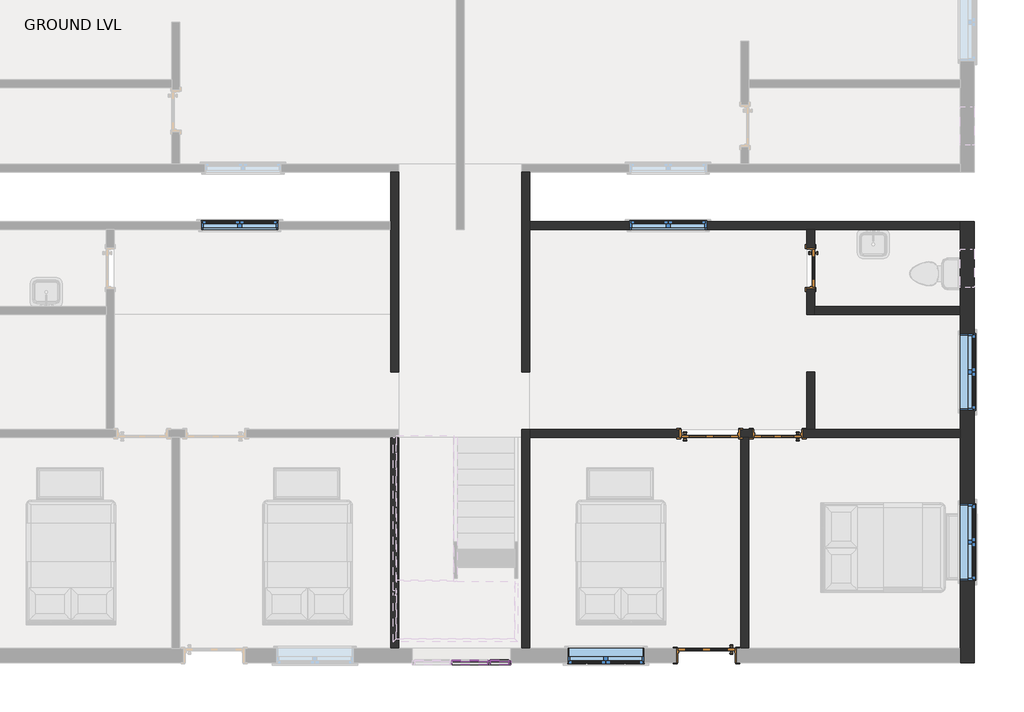
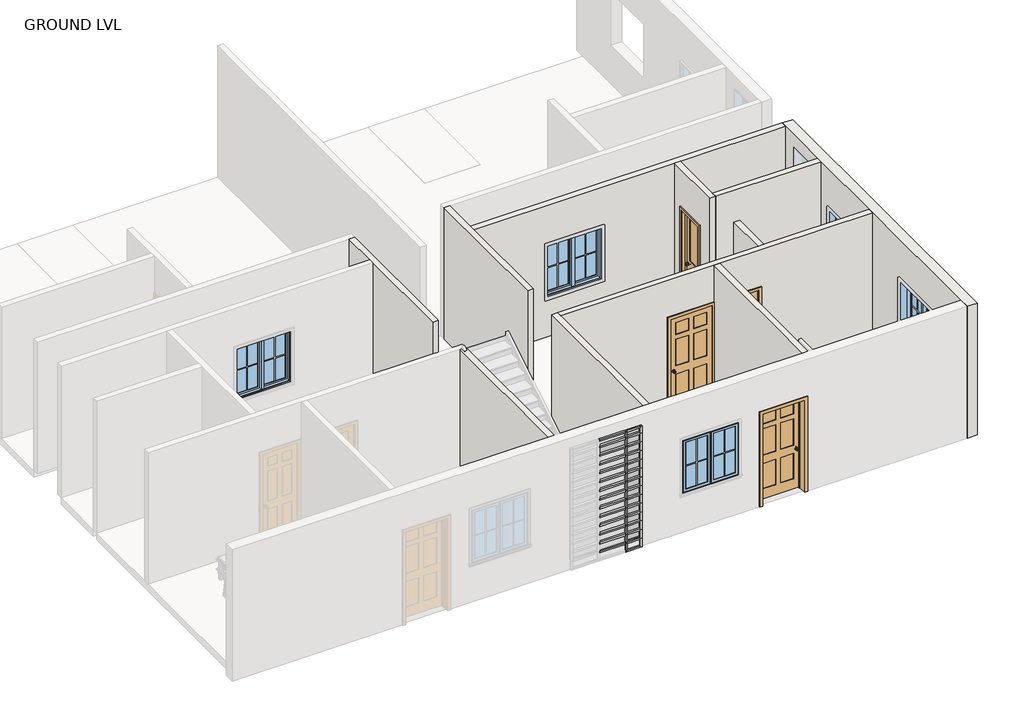
# One storey, part 2 of 4: 57 members, 15 plates, 11 walls, 5 windows, 4 doors.
"""IFC4 building model written with IfcOpenShell, lengths in millimetres."""

from ifc_helpers import new_model, si_unit, origin, origin_with_axes, place, context, project, spatial, polyline, outline, extrude, faceted_brep, transform, mapped, element, save
from components import door_596d7c92, door_d66ee888, door_c610b25b, door_c5239341, member_56b223d9, member_a59c64b1, member_06854975, member_b8e7570c, member_a67f877f, member_00eacae2, member_ff422208, member_dc11c383, system_panel_glazed_23b8b45c, system_panel_glazed_58d257f9, system_panel_glazed_e426d894, system_panel_glazed_822b3193, window_9200f5ac, window_c2c97eee

model = new_model("IFC4")

# Units and contexts
model_context = context("Model", 3, world=origin())
ifc_project = project(units=[si_unit("LENGTHUNIT", "METRE", prefix="MILLI")], contexts=[model_context])

# Site, building, storey
site = spatial("IfcSite", under=ifc_project)
building = spatial("IfcBuilding", under=site)
storey = spatial("IfcBuildingStorey", under=building, Name="GROUND LVL", Elevation=0.0)

# Doors
placement = place(None, origin())
door_shape = door_596d7c92(model_context)
element("IfcDoor", 1, ObjectType="Door-Interior-Single-2_Panel-Wood : 24\" x 84\"", at=placement, inside=storey, context=model_context, shape_type="MappedRepresentation", body=[
    mapped(door_shape, transform((1301.4612669, -1548.6593836, 0.0), x_axis=(0.0, -1.0, 0.0), y_axis=(1.0, 0.0, 0.0), z_axis=(0.0, 0.0, 1.0))),
])
door_2_shape = door_d66ee888(model_context)
element("IfcDoor", 2, ObjectType="Door-Interior-Single-6_Panel-Wood : 30\" x 84\"", at=placement, inside=storey, context=model_context, shape_type="MappedRepresentation", body=[
    mapped(door_2_shape, transform((777.5862669, -4180.7343836, 0.0), x_axis=(-1.0, 0.0, 0.0), y_axis=(0.0, -1.0, 0.0), z_axis=(0.0, 0.0, 1.0))),
])
door_3_shape = door_c610b25b(model_context)
element("IfcDoor", 3, ObjectType="Door-Interior-Single-6_Panel-Wood : 36\" x 84\"", at=placement, inside=storey, context=model_context, shape_type="MappedRepresentation", body=[
    mapped(door_3_shape, transform((-301.9137331, -4180.7343836, 0.0), x_axis=(1.0, 0.0, 0.0), y_axis=(0.0, 1.0, 0.0), z_axis=(0.0, 0.0, 1.0))),
])
door_4_shape = door_c5239341(model_context)
element("IfcDoor", 4, ObjectType="Door-Interior-Single-6_Panel-Wood : 36\" x 84\"", at=placement, inside=storey, context=model_context, shape_type="MappedRepresentation", body=[
    mapped(door_4_shape, transform((-352.7137331, -7704.9843836, 0.0), x_axis=(-1.0, 0.0, 0.0), y_axis=(0.0, -1.0, 0.0), z_axis=(0.0, 0.0, 1.0))),
])

# Members
member_shape = member_56b223d9(model_context)
element("IfcMember", 5, ObjectType="Rectangular Mullion : 1.5\" x 2.5\" rectangular", at=placement, inside=storey, context=model_context, shape_type="MappedRepresentation", body=[
    mapped(member_shape, transform((-3807.0334597, -7822.4593836, 0.0), x_axis=(1.0, 0.0, 0.0), y_axis=(0.0, -1.0, 0.0), z_axis=(0.0, 0.0, -1.0))),
])
element("IfcMember", 6, ObjectType="Rectangular Mullion : 1.5\" x 2.5\" rectangular", at=placement, inside=storey, context=model_context, shape_type="MappedRepresentation", body=[
    mapped(member_shape, transform((-3807.0334597, -7822.4593836, 203.2), x_axis=(1.0, 0.0, 0.0), y_axis=(0.0, -1.0, 0.0), z_axis=(0.0, 0.0, -1.0))),
])
element("IfcMember", 7, ObjectType="Rectangular Mullion : 1.5\" x 2.5\" rectangular", at=placement, inside=storey, context=model_context, shape_type="MappedRepresentation", body=[
    mapped(member_shape, transform((-3807.0334597, -7822.4593836, 406.4), x_axis=(1.0, 0.0, 0.0), y_axis=(0.0, -1.0, 0.0), z_axis=(0.0, 0.0, -1.0))),
])
element("IfcMember", 8, ObjectType="Rectangular Mullion : 1.5\" x 2.5\" rectangular", at=placement, inside=storey, context=model_context, shape_type="MappedRepresentation", body=[
    mapped(member_shape, transform((-3807.0334597, -7822.4593836, 609.6), x_axis=(1.0, 0.0, 0.0), y_axis=(0.0, -1.0, 0.0), z_axis=(0.0, 0.0, -1.0))),
])
element("IfcMember", 9, ObjectType="Rectangular Mullion : 1.5\" x 2.5\" rectangular", at=placement, inside=storey, context=model_context, shape_type="MappedRepresentation", body=[
    mapped(member_shape, transform((-3807.0334597, -7822.4593836, 812.8), x_axis=(1.0, 0.0, 0.0), y_axis=(0.0, -1.0, 0.0), z_axis=(0.0, 0.0, -1.0))),
])
element("IfcMember", 10, ObjectType="Rectangular Mullion : 1.5\" x 2.5\" rectangular", at=placement, inside=storey, context=model_context, shape_type="MappedRepresentation", body=[
    mapped(member_shape, transform((-3807.0334597, -7822.4593836, 1016.0), x_axis=(1.0, 0.0, 0.0), y_axis=(0.0, -1.0, 0.0), z_axis=(0.0, 0.0, -1.0))),
])
element("IfcMember", 11, ObjectType="Rectangular Mullion : 1.5\" x 2.5\" rectangular", at=placement, inside=storey, context=model_context, shape_type="MappedRepresentation", body=[
    mapped(member_shape, transform((-3807.0334597, -7822.4593836, 1219.2), x_axis=(1.0, 0.0, 0.0), y_axis=(0.0, -1.0, 0.0), z_axis=(0.0, 0.0, -1.0))),
])
element("IfcMember", 12, ObjectType="Rectangular Mullion : 1.5\" x 2.5\" rectangular", at=placement, inside=storey, context=model_context, shape_type="MappedRepresentation", body=[
    mapped(member_shape, transform((-3807.0334597, -7822.4593836, 1422.4), x_axis=(1.0, 0.0, 0.0), y_axis=(0.0, -1.0, 0.0), z_axis=(0.0, 0.0, -1.0))),
])
element("IfcMember", 13, ObjectType="Rectangular Mullion : 1.5\" x 2.5\" rectangular", at=placement, inside=storey, context=model_context, shape_type="MappedRepresentation", body=[
    mapped(member_shape, transform((-3807.0334597, -7822.4593836, 1625.6), x_axis=(1.0, 0.0, 0.0), y_axis=(0.0, -1.0, 0.0), z_axis=(0.0, 0.0, -1.0))),
])
element("IfcMember", 14, ObjectType="Rectangular Mullion : 1.5\" x 2.5\" rectangular", at=placement, inside=storey, context=model_context, shape_type="MappedRepresentation", body=[
    mapped(member_shape, transform((-3807.0334597, -7822.4593836, 1828.8), x_axis=(1.0, 0.0, 0.0), y_axis=(0.0, -1.0, 0.0), z_axis=(0.0, 0.0, -1.0))),
])
element("IfcMember", 15, ObjectType="Rectangular Mullion : 1.5\" x 2.5\" rectangular", at=placement, inside=storey, context=model_context, shape_type="MappedRepresentation", body=[
    mapped(member_shape, transform((-3807.0334597, -7822.4593836, 2032.0), x_axis=(1.0, 0.0, 0.0), y_axis=(0.0, -1.0, 0.0), z_axis=(0.0, 0.0, -1.0))),
])
element("IfcMember", 16, ObjectType="Rectangular Mullion : 1.5\" x 2.5\" rectangular", at=placement, inside=storey, context=model_context, shape_type="MappedRepresentation", body=[
    mapped(member_shape, transform((-3807.0334597, -7822.4593836, 2235.2), x_axis=(1.0, 0.0, 0.0), y_axis=(0.0, -1.0, 0.0), z_axis=(0.0, 0.0, -1.0))),
])
element("IfcMember", 17, ObjectType="Rectangular Mullion : 1.5\" x 2.5\" rectangular", at=placement, inside=storey, context=model_context, shape_type="MappedRepresentation", body=[
    mapped(member_shape, transform((-3807.0334597, -7822.4593836, 2438.4), x_axis=(1.0, 0.0, 0.0), y_axis=(0.0, -1.0, 0.0), z_axis=(0.0, 0.0, -1.0))),
])
member_2_shape = member_a59c64b1(model_context)
element("IfcMember", 18, ObjectType="Rectangular Mullion : 1.5\" x 2.5\" rectangular", at=placement, inside=storey, context=model_context, shape_type="MappedRepresentation", body=[
    mapped(member_2_shape, transform((-3807.0334597, -7822.4593836, 2641.6), x_axis=(1.0, 0.0, 0.0), y_axis=(0.0, -1.0, 0.0), z_axis=(0.0, 0.0, -1.0))),
])
member_3_shape = member_06854975(model_context)
element("IfcMember", 19, ObjectType="Rectangular Mullion : 1.5\" x 2.5\" rectangular", at=placement, inside=storey, context=model_context, shape_type="MappedRepresentation", body=[
    mapped(member_3_shape, transform((-3499.7513929, -7822.4593836, 2807.3826151), x_axis=(0.0, 0.0, 1.0), y_axis=(0.0, -1.0, 0.0), z_axis=(1.0, 0.0, 0.0))),
])
member_4_shape = member_b8e7570c(model_context)
element("IfcMember", 20, ObjectType="Rectangular Mullion : 1.5\" x 2.5\" rectangular", at=placement, inside=storey, context=model_context, shape_type="MappedRepresentation", body=[
    mapped(member_4_shape, transform((-3826.0834597, -7822.4593836, 203.2), x_axis=(0.0, 0.0, 1.0), y_axis=(0.0, -1.0, 0.0), z_axis=(1.0, 0.0, 0.0))),
])
element("IfcMember", 21, ObjectType="Rectangular Mullion : 1.5\" x 2.5\" rectangular", at=placement, inside=storey, context=model_context, shape_type="MappedRepresentation", body=[
    mapped(member_4_shape, transform((-3826.0834597, -7822.4593836, 406.4), x_axis=(0.0, 0.0, 1.0), y_axis=(0.0, -1.0, 0.0), z_axis=(1.0, 0.0, 0.0))),
])
element("IfcMember", 22, ObjectType="Rectangular Mullion : 1.5\" x 2.5\" rectangular", at=placement, inside=storey, context=model_context, shape_type="MappedRepresentation", body=[
    mapped(member_4_shape, transform((-3826.0834597, -7822.4593836, 609.6), x_axis=(0.0, 0.0, 1.0), y_axis=(0.0, -1.0, 0.0), z_axis=(1.0, 0.0, 0.0))),
])
element("IfcMember", 23, ObjectType="Rectangular Mullion : 1.5\" x 2.5\" rectangular", at=placement, inside=storey, context=model_context, shape_type="MappedRepresentation", body=[
    mapped(member_4_shape, transform((-3826.0834597, -7822.4593836, 812.8), x_axis=(0.0, 0.0, 1.0), y_axis=(0.0, -1.0, 0.0), z_axis=(1.0, 0.0, 0.0))),
])
element("IfcMember", 24, ObjectType="Rectangular Mullion : 1.5\" x 2.5\" rectangular", at=placement, inside=storey, context=model_context, shape_type="MappedRepresentation", body=[
    mapped(member_4_shape, transform((-3826.0834597, -7822.4593836, 1016.0), x_axis=(0.0, 0.0, 1.0), y_axis=(0.0, -1.0, 0.0), z_axis=(1.0, 0.0, 0.0))),
])
element("IfcMember", 25, ObjectType="Rectangular Mullion : 1.5\" x 2.5\" rectangular", at=placement, inside=storey, context=model_context, shape_type="MappedRepresentation", body=[
    mapped(member_4_shape, transform((-3826.0834597, -7822.4593836, 1219.2), x_axis=(0.0, 0.0, 1.0), y_axis=(0.0, -1.0, 0.0), z_axis=(1.0, 0.0, 0.0))),
])
element("IfcMember", 26, ObjectType="Rectangular Mullion : 1.5\" x 2.5\" rectangular", at=placement, inside=storey, context=model_context, shape_type="MappedRepresentation", body=[
    mapped(member_4_shape, transform((-3826.0834597, -7822.4593836, 1422.4), x_axis=(0.0, 0.0, 1.0), y_axis=(0.0, -1.0, 0.0), z_axis=(1.0, 0.0, 0.0))),
])
element("IfcMember", 27, ObjectType="Rectangular Mullion : 1.5\" x 2.5\" rectangular", at=placement, inside=storey, context=model_context, shape_type="MappedRepresentation", body=[
    mapped(member_4_shape, transform((-3826.0834597, -7822.4593836, 1625.6), x_axis=(0.0, 0.0, 1.0), y_axis=(0.0, -1.0, 0.0), z_axis=(1.0, 0.0, 0.0))),
])
element("IfcMember", 28, ObjectType="Rectangular Mullion : 1.5\" x 2.5\" rectangular", at=placement, inside=storey, context=model_context, shape_type="MappedRepresentation", body=[
    mapped(member_4_shape, transform((-3826.0834597, -7822.4593836, 1828.8), x_axis=(0.0, 0.0, 1.0), y_axis=(0.0, -1.0, 0.0), z_axis=(1.0, 0.0, 0.0))),
])
element("IfcMember", 29, ObjectType="Rectangular Mullion : 1.5\" x 2.5\" rectangular", at=placement, inside=storey, context=model_context, shape_type="MappedRepresentation", body=[
    mapped(member_4_shape, transform((-3826.0834597, -7822.4593836, 2032.0), x_axis=(0.0, 0.0, 1.0), y_axis=(0.0, -1.0, 0.0), z_axis=(1.0, 0.0, 0.0))),
])
element("IfcMember", 30, ObjectType="Rectangular Mullion : 1.5\" x 2.5\" rectangular", at=placement, inside=storey, context=model_context, shape_type="MappedRepresentation", body=[
    mapped(member_4_shape, transform((-3826.0834597, -7822.4593836, 2235.2), x_axis=(0.0, 0.0, 1.0), y_axis=(0.0, -1.0, 0.0), z_axis=(1.0, 0.0, 0.0))),
])
element("IfcMember", 31, ObjectType="Rectangular Mullion : 1.5\" x 2.5\" rectangular", at=placement, inside=storey, context=model_context, shape_type="MappedRepresentation", body=[
    mapped(member_4_shape, transform((-3826.0834597, -7822.4593836, 2438.4), x_axis=(0.0, 0.0, 1.0), y_axis=(0.0, -1.0, 0.0), z_axis=(1.0, 0.0, 0.0))),
])
element("IfcMember", 32, ObjectType="Rectangular Mullion : 1.5\" x 2.5\" rectangular", at=placement, inside=storey, context=model_context, shape_type="MappedRepresentation", body=[
    mapped(member_4_shape, transform((-3826.0834597, -7822.4593836, 2641.6), x_axis=(0.0, 0.0, 1.0), y_axis=(0.0, -1.0, 0.0), z_axis=(1.0, 0.0, 0.0))),
])
member_5_shape = member_a67f877f(model_context)
element("IfcMember", 33, ObjectType="Rectangular Mullion : 1.5\" x 2.5\" rectangular", at=placement, inside=storey, context=model_context, shape_type="MappedRepresentation", body=[
    mapped(member_5_shape, transform((-3826.0834597, -7822.4593836, 2807.3826151), x_axis=(0.0, 0.0, 1.0), y_axis=(0.0, -1.0, 0.0), z_axis=(1.0, 0.0, 0.0))),
])
element("IfcMember", 34, ObjectType="Rectangular Mullion : 1.5\" x 2.5\" rectangular", at=placement, inside=storey, context=model_context, shape_type="MappedRepresentation", body=[
    mapped(member_3_shape, transform((-3787.9834597, -7822.4593836, 0.0), x_axis=(0.0, 0.0, -1.0), y_axis=(0.0, -1.0, 0.0), z_axis=(-1.0, 0.0, 0.0))),
])
member_6_shape = member_00eacae2(model_context)
element("IfcMember", 35, ObjectType="Rectangular Mullion : 1.5\" x 2.5\" rectangular", at=placement, inside=storey, context=model_context, shape_type="MappedRepresentation", body=[
    mapped(member_6_shape, transform((-3499.7513929, -7822.4593836, 203.2), x_axis=(0.0, 0.0, 1.0), y_axis=(0.0, -1.0, 0.0), z_axis=(1.0, 0.0, 0.0))),
])
element("IfcMember", 36, ObjectType="Rectangular Mullion : 1.5\" x 2.5\" rectangular", at=placement, inside=storey, context=model_context, shape_type="MappedRepresentation", body=[
    mapped(member_6_shape, transform((-3499.7513929, -7822.4593836, 406.4), x_axis=(0.0, 0.0, 1.0), y_axis=(0.0, -1.0, 0.0), z_axis=(1.0, 0.0, 0.0))),
])
element("IfcMember", 37, ObjectType="Rectangular Mullion : 1.5\" x 2.5\" rectangular", at=placement, inside=storey, context=model_context, shape_type="MappedRepresentation", body=[
    mapped(member_6_shape, transform((-3499.7513929, -7822.4593836, 609.6), x_axis=(0.0, 0.0, 1.0), y_axis=(0.0, -1.0, 0.0), z_axis=(1.0, 0.0, 0.0))),
])
element("IfcMember", 38, ObjectType="Rectangular Mullion : 1.5\" x 2.5\" rectangular", at=placement, inside=storey, context=model_context, shape_type="MappedRepresentation", body=[
    mapped(member_6_shape, transform((-3499.7513929, -7822.4593836, 812.8), x_axis=(0.0, 0.0, 1.0), y_axis=(0.0, -1.0, 0.0), z_axis=(1.0, 0.0, 0.0))),
])
element("IfcMember", 39, ObjectType="Rectangular Mullion : 1.5\" x 2.5\" rectangular", at=placement, inside=storey, context=model_context, shape_type="MappedRepresentation", body=[
    mapped(member_6_shape, transform((-3499.7513929, -7822.4593836, 1016.0), x_axis=(0.0, 0.0, 1.0), y_axis=(0.0, -1.0, 0.0), z_axis=(1.0, 0.0, 0.0))),
])
element("IfcMember", 40, ObjectType="Rectangular Mullion : 1.5\" x 2.5\" rectangular", at=placement, inside=storey, context=model_context, shape_type="MappedRepresentation", body=[
    mapped(member_6_shape, transform((-3499.7513929, -7822.4593836, 1219.2), x_axis=(0.0, 0.0, 1.0), y_axis=(0.0, -1.0, 0.0), z_axis=(1.0, 0.0, 0.0))),
])
element("IfcMember", 41, ObjectType="Rectangular Mullion : 1.5\" x 2.5\" rectangular", at=placement, inside=storey, context=model_context, shape_type="MappedRepresentation", body=[
    mapped(member_6_shape, transform((-3499.7513929, -7822.4593836, 1422.4), x_axis=(0.0, 0.0, 1.0), y_axis=(0.0, -1.0, 0.0), z_axis=(1.0, 0.0, 0.0))),
])
element("IfcMember", 42, ObjectType="Rectangular Mullion : 1.5\" x 2.5\" rectangular", at=placement, inside=storey, context=model_context, shape_type="MappedRepresentation", body=[
    mapped(member_6_shape, transform((-3499.7513929, -7822.4593836, 1625.6), x_axis=(0.0, 0.0, 1.0), y_axis=(0.0, -1.0, 0.0), z_axis=(1.0, 0.0, 0.0))),
])
element("IfcMember", 43, ObjectType="Rectangular Mullion : 1.5\" x 2.5\" rectangular", at=placement, inside=storey, context=model_context, shape_type="MappedRepresentation", body=[
    mapped(member_6_shape, transform((-3499.7513929, -7822.4593836, 1828.8), x_axis=(0.0, 0.0, 1.0), y_axis=(0.0, -1.0, 0.0), z_axis=(1.0, 0.0, 0.0))),
])
element("IfcMember", 44, ObjectType="Rectangular Mullion : 1.5\" x 2.5\" rectangular", at=placement, inside=storey, context=model_context, shape_type="MappedRepresentation", body=[
    mapped(member_6_shape, transform((-3499.7513929, -7822.4593836, 2032.0), x_axis=(0.0, 0.0, 1.0), y_axis=(0.0, -1.0, 0.0), z_axis=(1.0, 0.0, 0.0))),
])
element("IfcMember", 45, ObjectType="Rectangular Mullion : 1.5\" x 2.5\" rectangular", at=placement, inside=storey, context=model_context, shape_type="MappedRepresentation", body=[
    mapped(member_6_shape, transform((-3499.7513929, -7822.4593836, 2235.2), x_axis=(0.0, 0.0, 1.0), y_axis=(0.0, -1.0, 0.0), z_axis=(1.0, 0.0, 0.0))),
])
element("IfcMember", 46, ObjectType="Rectangular Mullion : 1.5\" x 2.5\" rectangular", at=placement, inside=storey, context=model_context, shape_type="MappedRepresentation", body=[
    mapped(member_6_shape, transform((-3499.7513929, -7822.4593836, 2438.4), x_axis=(0.0, 0.0, 1.0), y_axis=(0.0, -1.0, 0.0), z_axis=(1.0, 0.0, 0.0))),
])
element("IfcMember", 47, ObjectType="Rectangular Mullion : 1.5\" x 2.5\" rectangular", at=placement, inside=storey, context=model_context, shape_type="MappedRepresentation", body=[
    mapped(member_6_shape, transform((-3499.7513929, -7822.4593836, 2641.6), x_axis=(0.0, 0.0, 1.0), y_axis=(0.0, -1.0, 0.0), z_axis=(1.0, 0.0, 0.0))),
])
member_7_shape = member_ff422208(model_context)
element("IfcMember", 48, ObjectType="Rectangular Mullion : 1.5\" x 2.5\" rectangular", at=placement, inside=storey, context=model_context, shape_type="MappedRepresentation", body=[
    mapped(member_7_shape, transform((-3461.6513929, -7822.4593836, 0.0), x_axis=(1.0, 0.0, 0.0), y_axis=(0.0, -1.0, 0.0), z_axis=(0.0, 0.0, -1.0))),
])
element("IfcMember", 49, ObjectType="Rectangular Mullion : 1.5\" x 2.5\" rectangular", at=placement, inside=storey, context=model_context, shape_type="MappedRepresentation", body=[
    mapped(member_7_shape, transform((-3461.6513929, -7822.4593836, 203.2), x_axis=(1.0, 0.0, 0.0), y_axis=(0.0, -1.0, 0.0), z_axis=(0.0, 0.0, -1.0))),
])
element("IfcMember", 50, ObjectType="Rectangular Mullion : 1.5\" x 2.5\" rectangular", at=placement, inside=storey, context=model_context, shape_type="MappedRepresentation", body=[
    mapped(member_7_shape, transform((-3461.6513929, -7822.4593836, 406.4), x_axis=(1.0, 0.0, 0.0), y_axis=(0.0, -1.0, 0.0), z_axis=(0.0, 0.0, -1.0))),
])
element("IfcMember", 51, ObjectType="Rectangular Mullion : 1.5\" x 2.5\" rectangular", at=placement, inside=storey, context=model_context, shape_type="MappedRepresentation", body=[
    mapped(member_7_shape, transform((-3461.6513929, -7822.4593836, 609.6), x_axis=(1.0, 0.0, 0.0), y_axis=(0.0, -1.0, 0.0), z_axis=(0.0, 0.0, -1.0))),
])
element("IfcMember", 52, ObjectType="Rectangular Mullion : 1.5\" x 2.5\" rectangular", at=placement, inside=storey, context=model_context, shape_type="MappedRepresentation", body=[
    mapped(member_7_shape, transform((-3461.6513929, -7822.4593836, 812.8), x_axis=(1.0, 0.0, 0.0), y_axis=(0.0, -1.0, 0.0), z_axis=(0.0, 0.0, -1.0))),
])
element("IfcMember", 53, ObjectType="Rectangular Mullion : 1.5\" x 2.5\" rectangular", at=placement, inside=storey, context=model_context, shape_type="MappedRepresentation", body=[
    mapped(member_7_shape, transform((-3461.6513929, -7822.4593836, 1016.0), x_axis=(1.0, 0.0, 0.0), y_axis=(0.0, -1.0, 0.0), z_axis=(0.0, 0.0, -1.0))),
])
element("IfcMember", 54, ObjectType="Rectangular Mullion : 1.5\" x 2.5\" rectangular", at=placement, inside=storey, context=model_context, shape_type="MappedRepresentation", body=[
    mapped(member_7_shape, transform((-3461.6513929, -7822.4593836, 1219.2), x_axis=(1.0, 0.0, 0.0), y_axis=(0.0, -1.0, 0.0), z_axis=(0.0, 0.0, -1.0))),
])
element("IfcMember", 55, ObjectType="Rectangular Mullion : 1.5\" x 2.5\" rectangular", at=placement, inside=storey, context=model_context, shape_type="MappedRepresentation", body=[
    mapped(member_7_shape, transform((-3461.6513929, -7822.4593836, 1422.4), x_axis=(1.0, 0.0, 0.0), y_axis=(0.0, -1.0, 0.0), z_axis=(0.0, 0.0, -1.0))),
])
element("IfcMember", 56, ObjectType="Rectangular Mullion : 1.5\" x 2.5\" rectangular", at=placement, inside=storey, context=model_context, shape_type="MappedRepresentation", body=[
    mapped(member_7_shape, transform((-3461.6513929, -7822.4593836, 1625.6), x_axis=(1.0, 0.0, 0.0), y_axis=(0.0, -1.0, 0.0), z_axis=(0.0, 0.0, -1.0))),
])
element("IfcMember", 57, ObjectType="Rectangular Mullion : 1.5\" x 2.5\" rectangular", at=placement, inside=storey, context=model_context, shape_type="MappedRepresentation", body=[
    mapped(member_7_shape, transform((-3461.6513929, -7822.4593836, 1828.8), x_axis=(1.0, 0.0, 0.0), y_axis=(0.0, -1.0, 0.0), z_axis=(0.0, 0.0, -1.0))),
])
element("IfcMember", 58, ObjectType="Rectangular Mullion : 1.5\" x 2.5\" rectangular", at=placement, inside=storey, context=model_context, shape_type="MappedRepresentation", body=[
    mapped(member_7_shape, transform((-3461.6513929, -7822.4593836, 2032.0), x_axis=(1.0, 0.0, 0.0), y_axis=(0.0, -1.0, 0.0), z_axis=(0.0, 0.0, -1.0))),
])
element("IfcMember", 59, ObjectType="Rectangular Mullion : 1.5\" x 2.5\" rectangular", at=placement, inside=storey, context=model_context, shape_type="MappedRepresentation", body=[
    mapped(member_7_shape, transform((-3461.6513929, -7822.4593836, 2235.2), x_axis=(1.0, 0.0, 0.0), y_axis=(0.0, -1.0, 0.0), z_axis=(0.0, 0.0, -1.0))),
])
element("IfcMember", 60, ObjectType="Rectangular Mullion : 1.5\" x 2.5\" rectangular", at=placement, inside=storey, context=model_context, shape_type="MappedRepresentation", body=[
    mapped(member_7_shape, transform((-3461.6513929, -7822.4593836, 2438.4), x_axis=(1.0, 0.0, 0.0), y_axis=(0.0, -1.0, 0.0), z_axis=(0.0, 0.0, -1.0))),
])
member_8_shape = member_dc11c383(model_context)
element("IfcMember", 61, ObjectType="Rectangular Mullion : 1.5\" x 2.5\" rectangular", at=placement, inside=storey, context=model_context, shape_type="MappedRepresentation", body=[
    mapped(member_8_shape, transform((-3461.6513929, -7822.4593836, 2641.6), x_axis=(1.0, 0.0, 0.0), y_axis=(0.0, -1.0, 0.0), z_axis=(0.0, 0.0, -1.0))),
])

# Plates
system_panel_glazed_shape = system_panel_glazed_23b8b45c(model_context)
element("IfcPlate", 62, ObjectType="System Panel : Glazed", at=placement, inside=storey, context=model_context, shape_type="MappedRepresentation", body=[
    mapped(system_panel_glazed_shape, transform((-4111.8334597, -7822.4593836, 2457.45), x_axis=(1.0, 0.0, 0.0), y_axis=(0.0, 1.0, 0.0), z_axis=(0.0, 0.0, 1.0))),
])
system_panel_glazed_2_shape = system_panel_glazed_58d257f9(model_context)
element("IfcPlate", 63, ObjectType="System Panel : Glazed", at=placement, inside=storey, context=model_context, shape_type="MappedRepresentation", body=[
    mapped(system_panel_glazed_2_shape, transform((-3643.8674263, -7822.4593836, 38.1), x_axis=(1.0, 0.0, 0.0), y_axis=(0.0, 1.0, 0.0), z_axis=(0.0, 0.0, 1.0))),
])
system_panel_glazed_3_shape = system_panel_glazed_e426d894(model_context)
element("IfcPlate", 64, ObjectType="System Panel : Glazed", at=placement, inside=storey, context=model_context, shape_type="MappedRepresentation", body=[
    mapped(system_panel_glazed_3_shape, transform((-3643.8674263, -7822.4593836, 222.25), x_axis=(1.0, 0.0, 0.0), y_axis=(0.0, 1.0, 0.0), z_axis=(0.0, 0.0, 1.0))),
])
element("IfcPlate", 65, ObjectType="System Panel : Glazed", at=placement, inside=storey, context=model_context, shape_type="MappedRepresentation", body=[
    mapped(system_panel_glazed_3_shape, transform((-3643.8674263, -7822.4593836, 425.45), x_axis=(1.0, 0.0, 0.0), y_axis=(0.0, 1.0, 0.0), z_axis=(0.0, 0.0, 1.0))),
])
element("IfcPlate", 66, ObjectType="System Panel : Glazed", at=placement, inside=storey, context=model_context, shape_type="MappedRepresentation", body=[
    mapped(system_panel_glazed_3_shape, transform((-3643.8674263, -7822.4593836, 831.85), x_axis=(1.0, 0.0, 0.0), y_axis=(0.0, 1.0, 0.0), z_axis=(0.0, 0.0, 1.0))),
])
element("IfcPlate", 67, ObjectType="System Panel : Glazed", at=placement, inside=storey, context=model_context, shape_type="MappedRepresentation", body=[
    mapped(system_panel_glazed_3_shape, transform((-3643.8674263, -7822.4593836, 1035.05), x_axis=(1.0, 0.0, 0.0), y_axis=(0.0, 1.0, 0.0), z_axis=(0.0, 0.0, 1.0))),
])
element("IfcPlate", 68, ObjectType="System Panel : Glazed", at=placement, inside=storey, context=model_context, shape_type="MappedRepresentation", body=[
    mapped(system_panel_glazed_3_shape, transform((-3643.8674263, -7822.4593836, 1441.45), x_axis=(1.0, 0.0, 0.0), y_axis=(0.0, 1.0, 0.0), z_axis=(0.0, 0.0, 1.0))),
])
element("IfcPlate", 69, ObjectType="System Panel : Glazed", at=placement, inside=storey, context=model_context, shape_type="MappedRepresentation", body=[
    mapped(system_panel_glazed_3_shape, transform((-3643.8674263, -7822.4593836, 1644.65), x_axis=(1.0, 0.0, 0.0), y_axis=(0.0, 1.0, 0.0), z_axis=(0.0, 0.0, 1.0))),
])
element("IfcPlate", 70, ObjectType="System Panel : Glazed", at=placement, inside=storey, context=model_context, shape_type="MappedRepresentation", body=[
    mapped(system_panel_glazed_3_shape, transform((-3643.8674263, -7822.4593836, 2051.05), x_axis=(1.0, 0.0, 0.0), y_axis=(0.0, 1.0, 0.0), z_axis=(0.0, 0.0, 1.0))),
])
element("IfcPlate", 71, ObjectType="System Panel : Glazed", at=placement, inside=storey, context=model_context, shape_type="MappedRepresentation", body=[
    mapped(system_panel_glazed_3_shape, transform((-3643.8674263, -7822.4593836, 2254.25), x_axis=(1.0, 0.0, 0.0), y_axis=(0.0, 1.0, 0.0), z_axis=(0.0, 0.0, 1.0))),
])
element("IfcPlate", 72, ObjectType="System Panel : Glazed", at=placement, inside=storey, context=model_context, shape_type="MappedRepresentation", body=[
    mapped(system_panel_glazed_3_shape, transform((-3643.8674263, -7822.4593836, 628.65), x_axis=(1.0, 0.0, 0.0), y_axis=(0.0, 1.0, 0.0), z_axis=(0.0, 0.0, 1.0))),
])
element("IfcPlate", 73, ObjectType="System Panel : Glazed", at=placement, inside=storey, context=model_context, shape_type="MappedRepresentation", body=[
    mapped(system_panel_glazed_3_shape, transform((-3643.8674263, -7822.4593836, 1238.25), x_axis=(1.0, 0.0, 0.0), y_axis=(0.0, 1.0, 0.0), z_axis=(0.0, 0.0, 1.0))),
])
element("IfcPlate", 74, ObjectType="System Panel : Glazed", at=placement, inside=storey, context=model_context, shape_type="MappedRepresentation", body=[
    mapped(system_panel_glazed_3_shape, transform((-3643.8674263, -7822.4593836, 1847.85), x_axis=(1.0, 0.0, 0.0), y_axis=(0.0, 1.0, 0.0), z_axis=(0.0, 0.0, 1.0))),
])
element("IfcPlate", 75, ObjectType="System Panel : Glazed", at=placement, inside=storey, context=model_context, shape_type="MappedRepresentation", body=[
    mapped(system_panel_glazed_3_shape, transform((-3643.8674263, -7822.4593836, 2457.45), x_axis=(1.0, 0.0, 0.0), y_axis=(0.0, 1.0, 0.0), z_axis=(0.0, 0.0, 1.0))),
])
system_panel_glazed_4_shape = system_panel_glazed_822b3193(model_context)
element("IfcPlate", 76, ObjectType="System Panel : Glazed", at=placement, inside=storey, context=model_context, shape_type="MappedRepresentation", body=[
    mapped(system_panel_glazed_4_shape, transform((-3643.8674263, -7822.4593836, 2660.65), x_axis=(1.0, 0.0, 0.0), y_axis=(0.0, 1.0, 0.0), z_axis=(0.0, 0.0, 1.0))),
])

# Walls
element("IfcWall", 77, ObjectType="Inner Wall 5\"", at=placement, inside=storey, context=model_context, shape_type="Brep", body=[
    faceted_brep([(-5369.2137331, -24.6593836, 0.0), (-5369.2137331, -812.0593836, 0.0), (-5369.2137331, -939.0593836, 0.0), (-5369.2137331, -3199.6593836, 0.0), (-5369.2137331, -3199.6593836, 3048.0), (-5369.2137331, -939.0593836, 3048.0), (-5369.2137331, -812.0593836, 3048.0), (-5369.2137331, -24.6593836, 3048.0), (-5242.2137331, -24.6593836, 0.0), (-5242.2137331, -24.6593836, 3048.0), (-5242.2137331, -3199.6593836, 3048.0), (-5242.2137331, -3199.6593836, 0.0)], [[[0, 1, 2, 3, 4, 5, 6, 7]], [[8, 9, 10, 11]], [[3, 2, 1, 0, 8, 11]], [[4, 3, 11, 10]], [[0, 7, 9, 8]], [[7, 6, 5, 4, 10, 9]]]),
])
element("IfcWall", 78, ObjectType="Inner Wall 5\"", at=placement, inside=storey, context=model_context, shape_type="Brep", body=[
    faceted_brep([(-3286.4137331, -24.6593836, 0.0), (-3286.4137331, -3199.6593836, 0.0), (-3286.4137331, -3199.6593836, 3048.0), (-3286.4137331, -24.6593836, 3048.0), (-3159.4137331, -24.6593836, 0.0), (-3159.4137331, -24.6593836, 3048.0), (-3159.4137331, -812.0593836, 3048.0), (-3159.4137331, -939.0593836, 3048.0), (-3159.4137331, -3199.6593836, 3048.0), (-3159.4137331, -3199.6593836, 0.0), (-3159.4137331, -939.0593836, 0.0), (-3159.4137331, -812.0593836, 0.0)], [[[0, 1, 2, 3]], [[4, 5, 6, 7, 8, 9, 10, 11]], [[1, 0, 4, 11, 10, 9]], [[2, 1, 9, 8]], [[0, 3, 5, 4]], [[3, 2, 8, 7, 6, 5]]]),
])
element("IfcWall", 79, ObjectType="Inner Wall 5\"", at=placement, inside=storey, context=model_context, shape_type="Brep", body=[
    faceted_brep([(3673.1862669, -812.0593836, 0.0), (-3159.4137331, -812.0593836, 0.0), (-3159.4137331, -812.0593836, 3048.0), (3673.1862669, -812.0593836, 3048.0), (-352.7137331, -812.0593836, 2133.6), (-1571.9137331, -812.0593836, 2133.6), (-1571.9137331, -812.0593836, 914.4), (-352.7137331, -812.0593836, 914.4), (3673.1862669, -939.0593836, 0.0), (3673.1862669, -939.0593836, 3048.0), (1361.7862669, -939.0593836, 3048.0), (1234.7862669, -939.0593836, 3048.0), (-3159.4137331, -939.0593836, 3048.0), (-3159.4137331, -939.0593836, 0.0), (1234.7862669, -939.0593836, 0.0), (1361.7862669, -939.0593836, 0.0), (-352.7137331, -939.0593836, 2133.6), (-352.7137331, -939.0593836, 914.4), (-1571.9137331, -939.0593836, 914.4), (-1571.9137331, -939.0593836, 2133.6)], [[[0, 1, 2, 3], [4, 5, 6, 7]], [[8, 9, 10, 11, 12, 13, 14, 15], [16, 17, 18, 19]], [[1, 0, 8, 15, 14, 13]], [[0, 3, 9, 8]], [[2, 1, 13, 12]], [[17, 16, 4, 7]], [[18, 17, 7, 6]], [[19, 18, 6, 5]], [[16, 19, 5, 4]], [[3, 2, 12, 11, 10, 9]]]),
])
element("IfcWall", 80, ObjectType="Inner Wall 5\"", at=placement, inside=storey, context=model_context, shape_type="Brep", body=[
    faceted_brep([(1234.7862669, -939.0593836, 3048.0), (1234.7862669, -939.0593836, 0.0), (1234.7862669, -1218.4593836, 0.0), (1234.7862669, -1218.4593836, 2159.0), (1234.7862669, -1878.8593836, 2159.0), (1234.7862669, -1878.8593836, 0.0), (1234.7862669, -2285.2593836, 0.0), (1234.7862669, -2285.2593836, 3048.0), (1361.7862669, -939.0593836, 0.0), (1361.7862669, -939.0593836, 3048.0), (1361.7862669, -2158.2593836, 3048.0), (1361.7862669, -2285.2593836, 3048.0), (1361.7862669, -2285.2593836, 0.0), (1361.7862669, -2158.2593836, 0.0), (1361.7862669, -1878.8593836, 0.0), (1361.7862669, -1878.8593836, 2159.0), (1361.7862669, -1218.4593836, 2159.0), (1361.7862669, -1218.4593836, 0.0)], [[[0, 1, 2, 3, 4, 5, 6, 7]], [[8, 9, 10, 11, 12, 13, 14, 15, 16, 17]], [[1, 8, 17, 2]], [[12, 6, 5, 14, 13]], [[1, 0, 9, 8]], [[7, 6, 12, 11]], [[4, 15, 14, 5]], [[15, 4, 3, 16]], [[16, 3, 2, 17]], [[0, 7, 11, 10, 9]]]),
])
element("IfcWall", 81, ObjectType="Inner Wall 5\"", at=placement, inside=storey, context=model_context, shape_type="SweptSolid", body=[
    extrude(outline(polyline([(3673.1862669, -2285.2593836), (1361.7862669, -2285.2593836), (1361.7862669, -2158.2593836), (3673.1862669, -2158.2593836), (3673.1862669, -2285.2593836)])), origin_with_axes(), (0.0, 0.0, 1.0), 3048.0),
])
element("IfcWall", 82, ObjectType="Inner Wall 5\"", at=placement, inside=storey, context=model_context, shape_type="SweptSolid", body=[
    extrude(outline(polyline([(-5242.2137331, -4241.0593836), (-5242.2137331, -7593.8593836), (-5369.2137331, -7593.8593836), (-5369.2137331, -4241.0593836), (-5242.2137331, -4241.0593836)])), origin_with_axes(), (0.0, 0.0, 1.0), 3048.0),
])
element("IfcWall", 83, ObjectType="Inner Wall 5\"", at=placement, inside=storey, context=model_context, shape_type="Brep", body=[
    faceted_brep([(-3159.4137331, -7593.8593836, 0.0), (-3159.4137331, -4241.0593836, 0.0), (-3159.4137331, -4114.0593836, 0.0), (-3159.4137331, -4114.0593836, 3048.0), (-3159.4137331, -4241.0593836, 3048.0), (-3159.4137331, -7593.8593836, 3048.0), (-3286.4137331, -7593.8593836, 0.0), (-3286.4137331, -7593.8593836, 3048.0), (-3286.4137331, -4114.0593836, 3048.0), (-3286.4137331, -4114.0593836, 0.0)], [[[0, 1, 2, 3, 4, 5]], [[6, 7, 8, 9]], [[2, 1, 0, 6, 9]], [[0, 5, 7, 6]], [[3, 2, 9, 8]], [[5, 4, 3, 8, 7]]]),
])
element("IfcWall", 84, ObjectType="Inner Wall 5\"", at=placement, inside=storey, context=model_context, shape_type="Brep", body=[
    faceted_brep([(-3159.4137331, -4241.0593836, 3048.0), (-3159.4137331, -4241.0593836, 0.0), (-784.5137331, -4241.0593836, 0.0), (-784.5137331, -4241.0593836, 2159.0), (180.6862669, -4241.0593836, 2159.0), (180.6862669, -4241.0593836, 0.0), (193.3862669, -4241.0593836, 0.0), (320.3862669, -4241.0593836, 0.0), (371.1862669, -4241.0593836, 0.0), (371.1862669, -4241.0593836, 2159.0), (1183.9862669, -4241.0593836, 2159.0), (1183.9862669, -4241.0593836, 0.0), (3673.1862669, -4241.0593836, 0.0), (3673.1862669, -4241.0593836, 3048.0), (320.3862669, -4241.0593836, 3048.0), (193.3862669, -4241.0593836, 3048.0), (-3159.4137331, -4114.0593836, 0.0), (-3159.4137331, -4114.0593836, 3048.0), (1234.7862669, -4114.0593836, 3048.0), (1361.7862669, -4114.0593836, 3048.0), (3673.1862669, -4114.0593836, 3048.0), (3673.1862669, -4114.0593836, 0.0), (1361.7862669, -4114.0593836, 0.0), (1234.7862669, -4114.0593836, 0.0), (1183.9862669, -4114.0593836, 0.0), (1183.9862669, -4114.0593836, 2159.0), (371.1862669, -4114.0593836, 2159.0), (371.1862669, -4114.0593836, 0.0), (180.6862669, -4114.0593836, 0.0), (180.6862669, -4114.0593836, 2159.0), (-784.5137331, -4114.0593836, 2159.0), (-784.5137331, -4114.0593836, 0.0)], [[[0, 1, 2, 3, 4, 5, 6, 7, 8, 9, 10, 11, 12, 13, 14, 15]], [[16, 17, 18, 19, 20, 21, 22, 23, 24, 25, 26, 27, 28, 29, 30, 31]], [[1, 16, 31, 2]], [[21, 12, 11, 24, 23, 22]], [[5, 28, 27, 8, 7, 6]], [[1, 0, 17, 16]], [[13, 12, 21, 20]], [[4, 29, 28, 5]], [[29, 4, 3, 30]], [[30, 3, 2, 31]], [[26, 9, 8, 27]], [[9, 26, 25, 10]], [[10, 25, 24, 11]], [[0, 15, 14, 13, 20, 19, 18, 17]]]),
])
element("IfcWall", 85, ObjectType="Inner Wall 5\"", at=placement, inside=storey, context=model_context, shape_type="SweptSolid", body=[
    extrude(outline(polyline([(320.3862669, -4241.0593836), (320.3862669, -7593.8593836), (193.3862669, -7593.8593836), (193.3862669, -4241.0593836), (320.3862669, -4241.0593836)])), origin_with_axes(), (0.0, 0.0, 1.0), 3048.0),
])
element("IfcWall", 86, ObjectType="Inner Wall 5\"", at=placement, inside=storey, context=model_context, shape_type="SweptSolid", body=[
    extrude(outline(polyline([(1361.7862669, -3199.6593836), (1361.7862669, -4114.0593836), (1234.7862669, -4114.0593836), (1234.7862669, -3199.6593836), (1361.7862669, -3199.6593836)])), origin_with_axes(), (0.0, 0.0, 1.0), 3048.0),
])
element("IfcWall", 87, ObjectType="outer wall 9\"", at=placement, inside=storey, context=model_context, shape_type="Brep", body=[
    faceted_brep([(3901.7862669, -7822.4593836, 0.0), (3901.7862669, -812.0593836, 0.0), (3901.7862669, -812.0593836, 3048.0), (3901.7862669, -7822.4593836, 3048.0), (3901.7862669, -3809.2593836, 2133.6), (3901.7862669, -2590.0593836, 2133.6), (3901.7862669, -2590.0593836, 914.4), (3901.7862669, -3809.2593836, 914.4), (3901.7862669, -6514.3593836, 2133.6), (3901.7862669, -5295.1593836, 2133.6), (3901.7862669, -5295.1593836, 914.4), (3901.7862669, -6514.3593836, 914.4), (3901.7862669, -1853.4593836, 2743.2), (3901.7862669, -1243.8593836, 2743.2), (3901.7862669, -1243.8593836, 2133.6), (3901.7862669, -1853.4593836, 2133.6), (3673.1862669, -7822.4593836, 0.0), (3673.1862669, -7822.4593836, 3048.0), (3673.1862669, -7593.8593836, 3048.0), (3673.1862669, -4241.0593836, 3048.0), (3673.1862669, -4114.0593836, 3048.0), (3673.1862669, -2285.2593836, 3048.0), (3673.1862669, -2158.2593836, 3048.0), (3673.1862669, -939.0593836, 3048.0), (3673.1862669, -812.0593836, 3048.0), (3673.1862669, -812.0593836, 0.0), (3673.1862669, -939.0593836, 0.0), (3673.1862669, -2158.2593836, 0.0), (3673.1862669, -2285.2593836, 0.0), (3673.1862669, -4114.0593836, 0.0), (3673.1862669, -4241.0593836, 0.0), (3673.1862669, -7593.8593836, 0.0), (3673.1862669, -3809.2593836, 2133.6), (3673.1862669, -3809.2593836, 914.4), (3673.1862669, -2590.0593836, 914.4), (3673.1862669, -2590.0593836, 2133.6), (3673.1862669, -6514.3593836, 2133.6), (3673.1862669, -6514.3593836, 914.4), (3673.1862669, -5295.1593836, 914.4), (3673.1862669, -5295.1593836, 2133.6), (3673.1862669, -1853.4593836, 2743.2), (3673.1862669, -1853.4593836, 2133.6), (3673.1862669, -1243.8593836, 2133.6), (3673.1862669, -1243.8593836, 2743.2)], [[[0, 1, 2, 3], [4, 5, 6, 7], [8, 9, 10, 11], [12, 13, 14, 15]], [[16, 17, 18, 19, 20, 21, 22, 23, 24, 25, 26, 27, 28, 29, 30, 31], [32, 33, 34, 35], [36, 37, 38, 39], [40, 41, 42, 43]], [[1, 0, 16, 31, 30, 29, 28, 27, 26, 25]], [[0, 3, 17, 16]], [[2, 1, 25, 24]], [[33, 32, 4, 7]], [[34, 33, 7, 6]], [[35, 34, 6, 5]], [[32, 35, 5, 4]], [[37, 36, 8, 11]], [[38, 37, 11, 10]], [[39, 38, 10, 9]], [[36, 39, 9, 8]], [[41, 40, 12, 15]], [[42, 41, 15, 14]], [[43, 42, 14, 13]], [[40, 43, 13, 12]], [[3, 2, 24, 23, 22, 21, 20, 19, 18, 17]]]),
])

# Windows
window_shape = window_9200f5ac(model_context)
element("IfcWindow", 88, ObjectType="Window-Casement-Double : 48\" x 48\"", at=placement, inside=storey, context=model_context, shape_type="MappedRepresentation", body=[
    mapped(window_shape, transform((3787.4862669, -3199.6593836, 0.0), x_axis=(0.0, -1.0, 0.0), y_axis=(1.0, 0.0, 0.0), z_axis=(0.0, 0.0, 1.0))),
])
element("IfcWindow", 89, ObjectType="Window-Casement-Double : 48\" x 48\"", at=placement, inside=storey, context=model_context, shape_type="MappedRepresentation", body=[
    mapped(window_shape, transform((3787.4862669, -5904.7593836, 0.0), x_axis=(0.0, -1.0, 0.0), y_axis=(1.0, 0.0, 0.0), z_axis=(0.0, 0.0, 1.0))),
])
element("IfcWindow", 90, ObjectType="Window-Casement-Double : 48\" x 48\"", at=placement, inside=storey, context=model_context, shape_type="MappedRepresentation", body=[
    mapped(window_shape, transform((-1952.9137331, -7708.1593836, 0.0), x_axis=(-1.0, 0.0, 0.0), y_axis=(0.0, -1.0, 0.0), z_axis=(0.0, 0.0, 1.0))),
])
window_2_shape = window_c2c97eee(model_context)
element("IfcWindow", 91, ObjectType="Window-Casement-Double : 48\" x 48\"", at=placement, inside=storey, context=model_context, shape_type="MappedRepresentation", body=[
    mapped(window_2_shape, transform((-7769.5137331, -875.5593836, 0.0), x_axis=(1.0, 0.0, 0.0), y_axis=(0.0, 1.0, 0.0), z_axis=(0.0, 0.0, 1.0))),
])
element("IfcWindow", 92, ObjectType="Window-Casement-Double : 48\" x 48\"", at=placement, inside=storey, context=model_context, shape_type="MappedRepresentation", body=[
    mapped(window_2_shape, transform((-962.3137331, -875.5593836, 0.0), x_axis=(1.0, 0.0, 0.0), y_axis=(0.0, 1.0, 0.0), z_axis=(0.0, 0.0, 1.0))),
])

save(model, "model.ifc")

# Revit data of these elements
# Type "Door-Interior-Single-2_Panel-Wood : 24\" x 84\""
#   Type Mark = "10"
#   Assembly Code = "C1020300"
#   Analytic Construction = "Wooden"
#   Top Rail = 0' - 4 11/16"
#   Thickness = 0' - 1 3/8"
#   Thermal Resistance (R) = 2.5876 (h·ft²·°F)/BTU
#   Swing Angle [instance default] = 90.00°
#   Stiles = 0' - 4 3/4"
#   Rough Width = 2' - 2"
#   Rough Height = 7' - 1"
#   Lock Rail = 0' - 7 1/2"
#   Height = 7' - 0"
#   Width = 2' - 0"
#   Heat Transfer Coefficient (U) = 0.3865 BTU/(h·ft²·°F)
#   Bottom Rail = 0' - 9 1/8"
#   Trim Material = Cherry
#   Panel Material = Cherry
#   Frame Material = Cherry
#   Door Handle Material = Aluminum
#   Visual Light Transmittance = 0
#   Solar Heat Gain Coefficient = 0
#   Wall Closure = (empty or 0)
#   Function = (empty or 0)
# Type "Door-Interior-Single-6_Panel-Wood : 30\" x 84\""
#   Type Mark = "9"
#   Assembly Code = "C1020300"
#   Analytic Construction = "Wooden"
#   Top Rail = 0' - 4 11/16"
#   Top Panel = 0' - 8"
#   Thickness = 0' - 1 3/8"
#   Thermal Resistance (R) = 2.5876 (h·ft²·°F)/BTU
#   Swing Angle [instance default] = 90.00°
#   Stiles = 0' - 4 3/4"
#   Rough Width = 2' - 8"
#   Rough Height = 7' - 1"
#   Mullion = 0' - 4 1/2"
#   Lock Rail = 0' - 7 1/2"
#   Intermediate Rail = 0' - 4 1/2"
#   Height = 7' - 0"
#   Width = 2' - 6"
#   Heat Transfer Coefficient (U) = 0.3865 BTU/(h·ft²·°F)
#   Bottom Rail = 0' - 9 1/8"
#   Trim Material = Cherry
#   Panel Material = Cherry
#   Frame Material = Cherry
#   Door Handle Material = Aluminum
#   Visual Light Transmittance = 0
#   Solar Heat Gain Coefficient = 0
#   Wall Closure = (empty or 0)
#   Function = (empty or 0)
# Type "Door-Interior-Single-6_Panel-Wood : 36\" x 84\""
#   Type Mark = "8"
#   Assembly Code = "C1020300"
#   Analytic Construction = "Wooden"
#   Top Rail = 0' - 4 11/16"
#   Top Panel = 0' - 11"
#   Thickness = 0' - 1 3/8"
#   Thermal Resistance (R) = 2.5876 (h·ft²·°F)/BTU
#   Swing Angle [instance default] = 90.00°
#   Stiles = 0' - 4 3/4"
#   Rough Width = 3' - 2"
#   Rough Height = 7' - 1"
#   Mullion = 0' - 4 1/2"
#   Lock Rail = 0' - 7 1/2"
#   Intermediate Rail = 0' - 4 1/2"
#   Height = 7' - 0"
#   Width = 3' - 0"
#   Heat Transfer Coefficient (U) = 0.3865 BTU/(h·ft²·°F)
#   Bottom Rail = 0' - 9 1/8"
#   Trim Material = Cherry
#   Panel Material = Cherry
#   Frame Material = Cherry
#   Door Handle Material = Aluminum
#   Visual Light Transmittance = 0
#   Solar Heat Gain Coefficient = 0
#   Wall Closure = (empty or 0)
#   Function = (empty or 0)
# Type "Rectangular Mullion : 1.5\" x 2.5\" rectangular"
#   built-in parameter 1007304 = 0.208333 (stored number, unit not read)
#   built-in parameter 1007301 = 0.0625 (stored number, unit not read)
#   built-in parameter 1007300 = 0.0625 (stored number, unit not read)
# Type "System Panel : Glazed"
#   Construction Type Id = "GSP4R"
#   Analytic Construction = "1/8 in Pilkington single glazing"
#   Visual Light Transmittance = 0.9
#   Solar Heat Gain Coefficient = 0.86
#   Heat Transfer Coefficient (U) = 1.18115 BTU/(h·ft²·°F)
#   Define Thermal Properties by = 1
# Type "Inner Wall 5\""
#   Assembly Code = "B2010"
#   Layers, outside or top first: 0' - 5" "wall paint" (function 1)
# Type "outer wall 9\""
#   Assembly Code = "B2010"
#   Layers, outside or top first: 0' - 9" "wall paint" (function 1)
# Type "Window-Casement-Double : 48\" x 48\""
#   Type Mark = "18"
#   Fire Rating = "0.5h"
#   Assembly Code = "B2020100"
#   Analytic Construction = "Double glazing - domestic"
#   Frame Extension [instance default] = 0' - 0 1/4"
#   Window Inset [instance default] = 0' - 0"
#   Wall Thickness [instance default] = 0' - 6"
#   Interior Wall Closure [instance default] = 0' - 2 1/4"
#   Half Width = 2' - 0"
#   Visual Light Transmittance = 0.81
#   Thermal Resistance (R) = 1.8146 (h·ft²·°F)/BTU
#   Solar Heat Gain Coefficient = 0.76
#   Rough Width = 4' - 0 1/2"
#   Rough Height = 4' - 0 1/2"
#   Height = 4' - 0"
#   Heat Transfer Coefficient (U) = 0.5511 BTU/(h·ft²·°F)
#   Exterior Wall Closure [instance default] = 0' - 1 1/4"
#   Extension Jamb [instance default] = 0' - 2 1/4"
#   Default Sill Height = 3' - 0"
#   Width = 4' - 0"
#   Muntin Visibility = yes
#   Interior Trim Visibility [instance default] = yes
#   Exterior Trim Visibility [instance default] = yes
#   Extension Jamb Visibility [instance default] = yes
#   Interior Trim Material = Wood - Stained
#   Muntin Pattern = Muntin Pattern_2x2 : Muntin Pattern_2x2
#   Interior Trim = Trim-Window-Interior-Flat : Picture Frame
#   Interior Frame Material = Wood - Stained
#   Glass Panel Material = Glass
#   Exterior Trim Material = Clad - White
#   Exterior Trim = Trim-Window-Exterior-Flat : with Sill
#   Exterior Frame Material = Clad - White
#   Wall Closure = (empty or 0)
# Element 1 (IfcDoor, "Door-Interior-Single-2_Panel-Wood : 24\" x 84\"")
#   Swing Angle = 90.00°
#   Phase Created = New Construction
#   Materials on its faces: "Cherry", "Aluminum"
# Element 2 (IfcDoor, "Door-Interior-Single-6_Panel-Wood : 30\" x 84\"")
#   Swing Angle = 90.00°
#   Phase Created = New Construction
#   Materials on its faces: "Cherry", "Aluminum"
# Elements 3, 4 (IfcDoor, "Door-Interior-Single-6_Panel-Wood : 36\" x 84\"")
#   Swing Angle = 90.00°
#   Phase Created = New Construction
#   Materials on its faces: "Cherry", "Aluminum"
# Elements 5, 6, 7, 8, 9, 10, 11, 12, 13, 14, 15, 16, 17, 18, 19, 20, 21, 22, 23, 24, 25, 26, 27, 28, 29, 30, 31, 32, 33, 34, 35, 36, 37, 38, 39, 40, 41, 42, 43, 44, 45, 46, 47, 48, 49, 50, 51, 52, 53, 54, 55, 56, 57, 58, 59, 60, 61 (IfcMember, "Rectangular Mullion : 1.5\" x 2.5\" rectangular")
#   Phase Created = New Construction
#   Materials on its faces: "Aluminum"
# Elements 62, 63, 64, 65, 66, 67, 68, 69, 70, 71, 72, 73, 74, 75, 76 (IfcPlate, "System Panel : Glazed")
#   Phase Created = New Construction
#   Materials on its faces: "Glass"
# Elements 77, 78, 80, 81, 82, 83, 84, 85, 86 (IfcWall, "Inner Wall 5\"")
#   Top Offset = 0' - 0"
#   Base Offset = 0' - 0"
#   Unconnected Height = 10' - 0"
#   wall height = 10' - 0"
#   Phase Created = New Construction
#   Base Constraint = GROUND LVL
#   Materials on its faces: "wall paint"
# Element 79 (IfcWall, "Inner Wall 5\"")
#   Top Offset = 0' - 0"
#   Base Offset = 0' - 0"
#   Unconnected Height = 10' - 0"
#   wall height = 10' - 0"
#   Phase Created = New Construction
#   Base Constraint = GROUND LVL
#   Materials on its faces: "wall paint", "Clad - White"
# Element 87 (IfcWall, "outer wall 9\"")
#   Top Offset = 0' - 0"
#   Base Offset = 0' - 0"
#   Unconnected Height = 10' - 0"
#   wall height = 10' - 0"
#   Phase Created = New Construction
#   Base Constraint = GROUND LVL
#   Materials on its faces: "wall paint", "Clad - White"
# Element 88 (IfcWindow, "Window-Casement-Double : 48\" x 48\"")
#   Mark = "9"
#   Window Inset = 0' - 0"
#   Interior Wall Closure = 0' - 2 1/4"
#   Frame Extension = 0' - 0 1/4"
#   Exterior Wall Closure = 0' - 1 1/4"
#   Interior Trim Visibility = yes
#   Exterior Trim Visibility = yes
#   Phase Created = New Construction
#   Materials on its faces: "Wood - Stained", "Glass", "Clad - White"
# Element 89 (IfcWindow, "Window-Casement-Double : 48\" x 48\"")
#   Mark = "10"
#   Window Inset = 0' - 0"
#   Interior Wall Closure = 0' - 2 1/4"
#   Frame Extension = 0' - 0 1/4"
#   Exterior Wall Closure = 0' - 1 1/4"
#   Interior Trim Visibility = yes
#   Exterior Trim Visibility = yes
#   Phase Created = New Construction
#   Materials on its faces: "Wood - Stained", "Glass", "Clad - White"
# Element 90 (IfcWindow, "Window-Casement-Double : 48\" x 48\"")
#   Mark = "11"
#   Window Inset = 0' - 0"
#   Interior Wall Closure = 0' - 2 1/4"
#   Frame Extension = 0' - 0 1/4"
#   Exterior Wall Closure = 0' - 1 1/4"
#   Interior Trim Visibility = yes
#   Exterior Trim Visibility = yes
#   Phase Created = New Construction
#   Materials on its faces: "Wood - Stained", "Glass", "Clad - White"
# Element 91 (IfcWindow, "Window-Casement-Double : 48\" x 48\"")
#   Mark = "15"
#   Window Inset = 0' - 0"
#   Interior Wall Closure = 0' - 2 1/4"
#   Frame Extension = 0' - 0 1/4"
#   Exterior Wall Closure = 0' - 1 1/4"
#   Interior Trim Visibility = yes
#   Exterior Trim Visibility = yes
#   Phase Created = New Construction
#   Materials on its faces: "Wood - Stained", "Glass", "Clad - White"
# Element 92 (IfcWindow, "Window-Casement-Double : 48\" x 48\"")
#   Mark = "17"
#   Window Inset = 0' - 0"
#   Interior Wall Closure = 0' - 2 1/4"
#   Frame Extension = 0' - 0 1/4"
#   Exterior Wall Closure = 0' - 1 1/4"
#   Interior Trim Visibility = yes
#   Exterior Trim Visibility = yes
#   Phase Created = New Construction
#   Materials on its faces: "Wood - Stained", "Glass", "Clad - White"
# Materials
#   "Cherry": class "Wood", colour RGB 226 177 128, transparency 0, Description = "Prunus Serotina", Cost = 0
#   "Aluminum": class "Metal", colour RGB 247 247 247, transparency 0, Description = "Aluminum 6061", Cost = 0
#   "wall paint": class "Generic", colour RGB 120 120 120, transparency 0, Cost = 0
#   "Wood - Stained": class "Wood", colour RGB 224 178 126, transparency 0, Cost = 0
#   "Glass": class "Glass", colour RGB 0 128 192, transparency 0.75, Description = "Soda Lime Glass", Cost = 0
#   "Clad - White": class "Wood", colour RGB 242 242 238, transparency 0, Cost = 0
